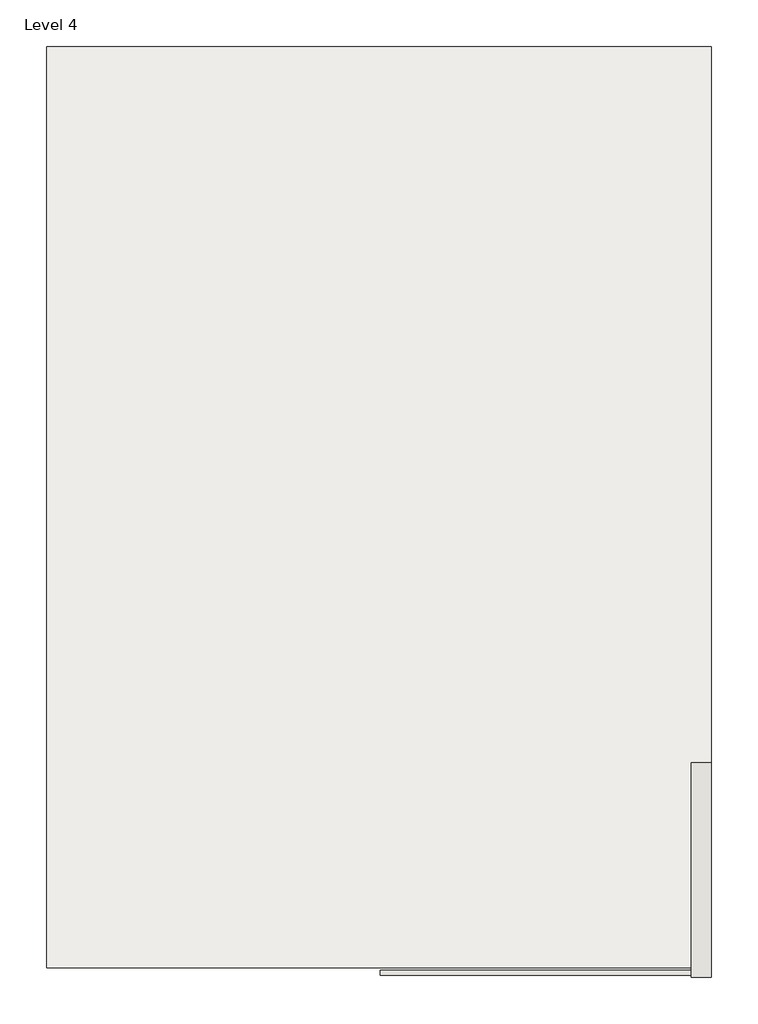
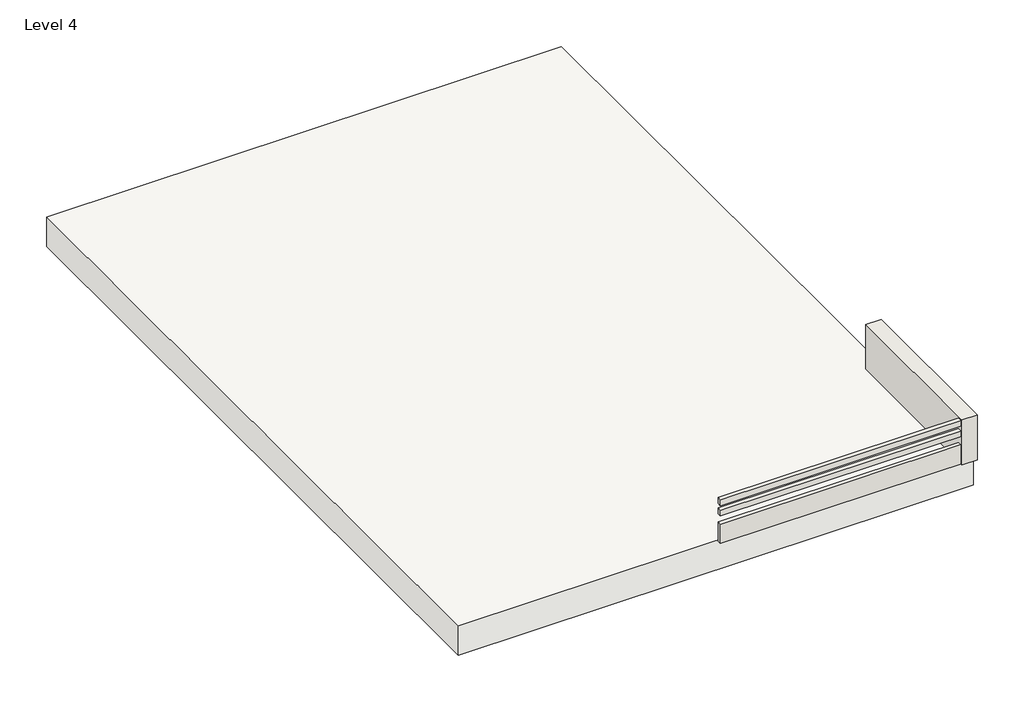
# One storey: 2 walls, 1 slab.
"""IFC4 building model written with IfcOpenShell, lengths in millimetres."""

from ifc_helpers import new_model, si_unit, frame, origin, place, context, project, spatial, polyline, outline, extrude, faceted_brep, transform, mapped, element, save
from components import walls_11_walls_11_77f6b4d3

model = new_model("IFC4")

# Units and contexts
model_context = context("Model", 3, world=origin())
ifc_project = project(units=[si_unit("LENGTHUNIT", "METRE", prefix="MILLI")], contexts=[model_context])

# Site, building, storey
site = spatial("IfcSite", under=ifc_project)
building = spatial("IfcBuilding", under=site)
storey = spatial("IfcBuildingStorey", under=building, Name="Level 4", Elevation=6096.0)

# Slab
placement = place(None, origin())
element("IfcSlab", 1, ObjectType="Generic Floor - 400mm", at=placement, inside=storey, context=model_context, shape_type="SweptSolid", body=[
    extrude(outline(polyline([(-5912.2996792, 1657.3086061), (-5912.2996792, -7490.0501996), (-12513.0996792, -7490.0501996), (-12513.0996792, 1657.3086061), (-5912.2996792, 1657.3086061)])), frame((0.0, 0.0, 5696.0), z_axis=(0.0, 0.0, 1.0), x_axis=(1.0, 0.0, 0.0)), (0.0, 0.0, 1.0), 400.0),
])

# Walls
element("IfcWall", 2, ObjectType="Generic - 9\"", at=placement, inside=storey, context=model_context, shape_type="Brep", body=[
    faceted_brep([(-6112.2996792, -5453.0913939, 6096.0), (-6112.2996792, -7586.6913939, 6096.0), (-6112.2996792, -7586.6913939, 6705.6), (-6112.2996792, -5453.0913939, 6705.6), (-6112.2996792, -5453.0913939, 6658.5115849), (-5912.2996792, -5453.0913939, 6096.0), (-5912.2996792, -5453.0913939, 6658.5115849), (-5912.2996792, -5453.0913939, 6705.6), (-5912.2996792, -7586.6913939, 6705.6), (-5912.2996792, -7586.6913939, 6096.0), (-5912.2996792, -5553.0913939, 6096.0)], [[[0, 1, 2, 3, 4]], [[5, 6, 7, 8, 9, 10]], [[1, 0, 5, 10, 9]], [[2, 1, 9, 8]], [[3, 2, 8, 7]], [[0, 4, 3, 7, 6, 5]]]),
])
walls_11_walls_11_shape = walls_11_walls_11_77f6b4d3(model_context)
element("IfcWall", 3, ObjectType="Walls 11 : Walls 11", at=placement, inside=storey, context=model_context, shape_type="MappedRepresentation", body=[
    mapped(walls_11_walls_11_shape, transform((0.0, 0.0, 0.0), x_axis=(1.0, 0.0, 0.0), y_axis=(0.0, 1.0, 0.0), z_axis=(0.0, 0.0, 1.0))),
])

save(model, "model.ifc")

# Revit data of these elements
# Type "Generic Floor - 400mm"
#   Function = 0
#   Layers, outside or top first: 400 mm no material (function 1)
# Type "Generic - 9\""
#   Layers, outside or top first: 200 mm no material (function 1)
# Element 1 (IfcSlab, "Generic Floor - 400mm")
#   Height Offset From Level = 0 mm
#   Phase Created = New Construction
#   Materials on its faces: "Default Roof"
# Element 2 (IfcWall, "Generic - 9\"")
#   Top Offset = 0 mm
#   Base Offset = 0 mm
#   Unconnected Height = 609.6 mm
#   wall height = 609.6 mm
#   Phase Created = New Construction
#   Base Constraint = Level 4
#   Materials on its faces: "Default Wall"
# Element 3 (IfcWall, "Walls 11 : Walls 11")
#   Phase Created = New Construction
#   Materials on its faces: "Default Wall"
# Materials
#   "Default Roof": colour RGB 80 80 80, transparency 0
#   "Default Wall": colour RGB 80 80 80, transparency 0
